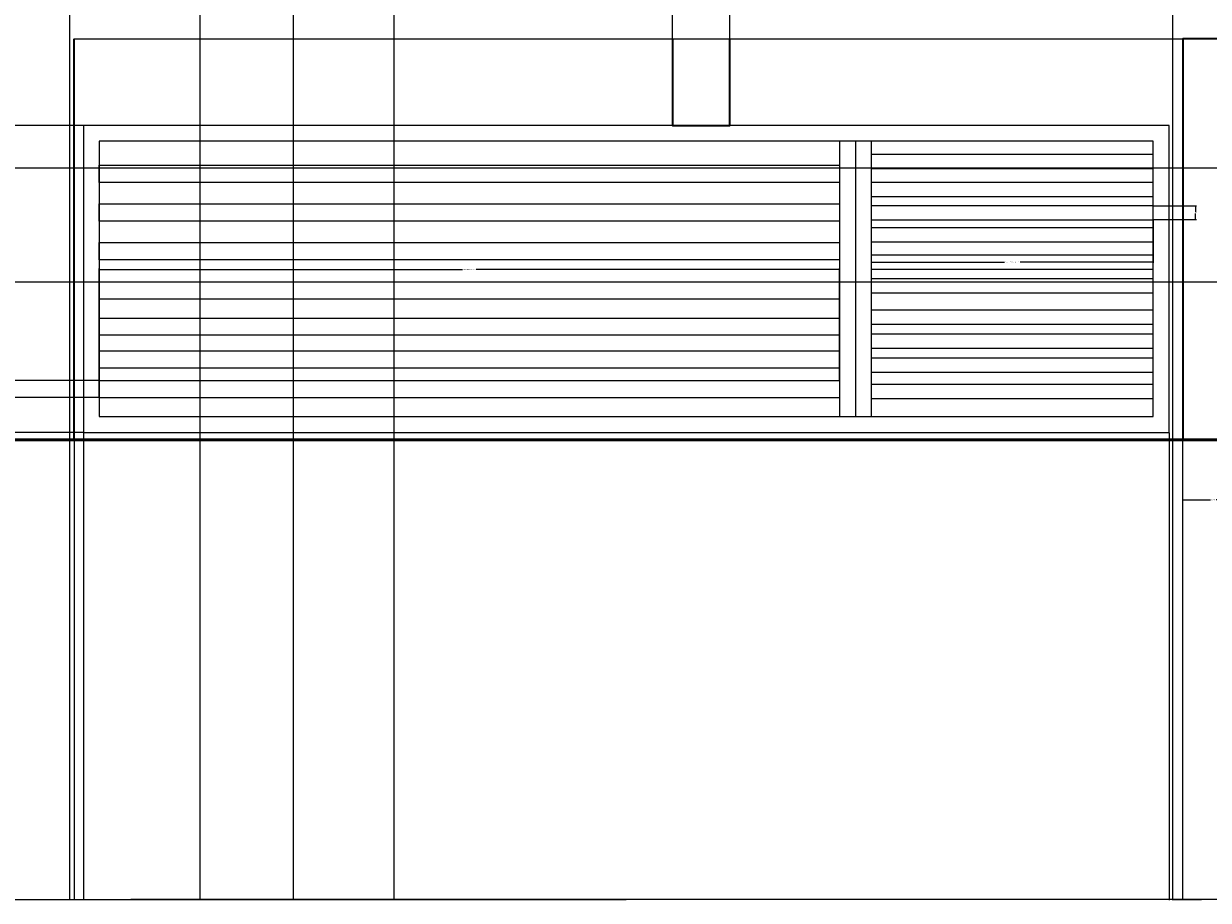
# Model space of a CAD drawing. Units: inches. Extents: x -8 to 554, y -200 to 499.
# Tile 3 of 12: x 214 to 439, y -200 to -34. Entities that reach past the tile are written whole.
import ezdxf

# ---------------------------------------------------------------- set-up
doc = ezdxf.new("R2010")
doc.units = ezdxf.units.IN
doc.header["$MEASUREMENT"] = 0
for name, color, linetype, lineweight in [('A-ANNO-DIMS', 2, 'Continuous', 18), ('A-COLS', 1, 'Continuous', 35), ('A-DOOR-GATE', 3, 'Continuous', 25), ('C-TOPO', 7, 'Continuous', 50)]:
    doc.layers.add(name, color=color, linetype=linetype, lineweight=lineweight)
doc.styles.get("Standard").update_dxf_attribs({"font": 'arial.ttf'})
doc.dimstyles.get("Standard").update_dxf_attribs({"dimtxt": 0.18, "dimasz": 0.18, "dimexe": 0.18, "dimexo": 0.0625, "dimgap": 0.09, "dimtad": 0, "dimtih": 1, "dimtoh": 1, "dimdec": 4, "dimzin": 0, "dimdsep": 46, "dimtxsty": 'Standard', "dimcen": 0.09, "dimadec": 0, "dimazin": 0, "dimtfac": 1, "dimtdec": 4, "dimtofl": 0, "dimtmove": 0, "dimatfit": 3, "dimfxl": 1, "dimtolj": 1, "dimtzin": 0, "dimarcsym": 0})

# ---------------------------------------------------------------- blocks, each defined once
blk = doc.blocks.new('GATE-PIER-ELEV')
blk.add_lwpolyline([(0, 76.14), (0, 0), (11.66, 0), (11.66, 76.14)])
blk = doc.blocks.new('GATE-SLAT-WIDE')
blk.add_lwpolyline([(0, 3.27), (140.62, 3.27), (140.62, 0), (0, 0)], close=True)
blk = doc.blocks.new('GATE-SLAT-NARROW')
blk.add_lwpolyline([(0, 0), (53.59, 0), (53.59, 2.66), (0, 2.66)], close=True)
blk = doc.blocks.new('*D12')
at = {"layer": 'A-ANNO-DIMS', "color": 0, "lineweight": -2, "transparency": 16777216}
for p, q in [((375.25, -70.8), (375.25, -78.95)), ((428.85, -70.8), (428.85, -78.95)), ((375.43, -78.77), (400.57, -78.77)), ((428.67, -78.77), (403.53, -78.77))]:
    blk.add_line(p, q, dxfattribs=at)
at = {"layer": 'A-ANNO-DIMS', "color": 0, "transparency": 16777216}
for points in [[(375.43, -78.74), (375.43, -78.8), (375.25, -78.77)], [(428.67, -78.74), (428.67, -78.8), (428.85, -78.77)]]:
    blk.add_solid(points, dxfattribs=at)
at = {"layer": 'Defpoints', "color": 0, "transparency": 16777216}
for p in [(375.25, -70.73), (428.85, -70.73), (428.85, -78.77)]:
    blk.add_point(p, dxfattribs=at)
at = {"layer": 'A-ANNO-DIMS', "color": 0, "transparency": 16777216, "insert": (402.05, -78.77), "char_height": 0.18, "attachment_point": 5}
blk.add_mtext('\\A1;NARROW SLAT 54 TYP.', dxfattribs=at)
blk = doc.blocks.new('*D13')
at = {"layer": 'A-ANNO-DIMS', "color": 0, "lineweight": -2, "transparency": 16777216}
for p, q in [((428.91, -68.08), (437.06, -68.08)), ((436.88, -68.26), (436.88, -69.22)), ((436.88, -70.55), (436.88, -69.59)), ((428.91, -70.73), (437.06, -70.73))]:
    blk.add_line(p, q, dxfattribs=at)
at = {"layer": 'A-ANNO-DIMS', "color": 0, "transparency": 16777216}
for points in [[(436.85, -68.26), (436.91, -68.26), (436.88, -68.08)], [(436.85, -70.55), (436.91, -70.55), (436.88, -70.73)]]:
    blk.add_solid(points, dxfattribs=at)
at = {"layer": 'Defpoints', "color": 0, "transparency": 16777216}
for p in [(428.85, -68.08), (436.88, -68.08), (428.85, -70.73)]:
    blk.add_point(p, dxfattribs=at)
at = {"layer": 'A-ANNO-DIMS', "color": 0, "transparency": 16777216, "insert": (436.88, -69.4), "char_height": 0.18, "attachment_point": 5}
blk.add_mtext('\\A1;3 TYP.', dxfattribs=at)
blk = doc.blocks.new('*D14')
at = {"layer": 'A-ANNO-DIMS', "color": 0, "lineweight": -2, "transparency": 16777216}
for p, q in [((228.63, -101.2), (228.63, -79.99)), ((228.81, -80.17), (297.63, -80.17)), ((369.07, -80.17), (300.26, -80.17)), ((369.25, -101.2), (369.25, -79.99))]:
    blk.add_line(p, q, dxfattribs=at)
at = {"layer": 'A-ANNO-DIMS', "color": 0, "transparency": 16777216}
for points in [[(228.81, -80.14), (228.81, -80.2), (228.63, -80.17)], [(369.07, -80.14), (369.07, -80.2), (369.25, -80.17)]]:
    blk.add_solid(points, dxfattribs=at)
at = {"layer": 'Defpoints', "color": 0, "transparency": 16777216}
for p in [(369.25, -80.17), (228.63, -101.26), (369.25, -101.26)]:
    blk.add_point(p, dxfattribs=at)
at = {"layer": 'A-ANNO-DIMS', "color": 0, "transparency": 16777216, "insert": (298.94, -80.17), "char_height": 0.18, "attachment_point": 5}
blk.add_mtext('\\A1;WIDE SLAT 141 TYP.', dxfattribs=at)
blk = doc.blocks.new('*D15')
at = {"layer": 'A-ANNO-DIMS', "color": 0, "lineweight": -2, "transparency": 16777216}
for p, q in [((228.57, -101.26), (207.36, -101.26)), ((207.54, -101.44), (207.54, -102.71)), ((207.54, -104.35), (207.54, -103.08)), ((228.57, -104.53), (207.36, -104.53))]:
    blk.add_line(p, q, dxfattribs=at)
at = {"layer": 'A-ANNO-DIMS', "color": 0, "transparency": 16777216}
for points in [[(207.51, -101.44), (207.57, -101.44), (207.54, -101.26)], [(207.51, -104.35), (207.57, -104.35), (207.54, -104.53)]]:
    blk.add_solid(points, dxfattribs=at)
at = {"layer": 'Defpoints', "color": 0, "transparency": 16777216}
for p in [(207.54, -101.26), (228.63, -101.26), (228.63, -104.53)]:
    blk.add_point(p, dxfattribs=at)
at = {"layer": 'A-ANNO-DIMS', "color": 0, "transparency": 16777216, "insert": (207.54, -102.9), "char_height": 0.18, "attachment_point": 5}
blk.add_mtext('\\A1;3 TYP.', dxfattribs=at)
blk = doc.blocks.new('*D29')
at = {"layer": 'A-ANNO-DIMS', "color": 0, "lineweight": -2, "transparency": 16777216}
for p, q in [((434.42, -112.58), (434.42, -124.12)), ((446.09, -112.58), (446.09, -124.12)), ((434.6, -123.94), (439.73, -123.94)), ((445.91, -123.94), (440.77, -123.94))]:
    blk.add_line(p, q, dxfattribs=at)
at = {"layer": 'A-ANNO-DIMS', "color": 0, "transparency": 16777216}
for points in [[(434.6, -123.91), (434.6, -123.97), (434.42, -123.94)], [(445.91, -123.91), (445.91, -123.97), (446.09, -123.94)]]:
    blk.add_solid(points, dxfattribs=at)
at = {"layer": 'Defpoints', "color": 0, "transparency": 16777216}
for p in [(434.42, -112.52), (446.09, -112.52), (434.42, -123.94)]:
    blk.add_point(p, dxfattribs=at)
at = {"layer": 'A-ANNO-DIMS', "color": 0, "transparency": 16777216, "insert": (440.25, -123.94), "char_height": 0.18, "attachment_point": 5}
blk.add_mtext('\\A1;12 TYP.', dxfattribs=at)
blk = doc.blocks.new('*D31')
at = {"layer": 'A-ANNO-DIMS', "color": 0, "lineweight": -2, "transparency": 16777216}
for p, q in [((24.34, 127.42), (24.34, -199.97)), ((453.32, -30.73), (453.32, -199.97)), ((24.52, -199.79), (238.54, -199.79)), ((453.14, -199.79), (239.12, -199.79))]:
    blk.add_line(p, q, dxfattribs=at)
at = {"layer": 'A-ANNO-DIMS', "color": 0, "transparency": 16777216}
for points in [[(24.52, -199.76), (24.52, -199.82), (24.34, -199.79)], [(453.14, -199.76), (453.14, -199.82), (453.32, -199.79)]]:
    blk.add_solid(points, dxfattribs=at)
at = {"layer": 'Defpoints', "color": 0, "transparency": 16777216}
for p in [(24.34, 127.48), (453.32, -30.67), (453.32, -199.79)]:
    blk.add_point(p, dxfattribs=at)
at = {"layer": 'A-ANNO-DIMS', "color": 0, "transparency": 16777216, "insert": (238.83, -199.79), "char_height": 0.18, "attachment_point": 5}
blk.add_mtext('\\A1;429', dxfattribs=at)
blk = doc.blocks.new('*D32')
at = {"layer": 'A-ANNO-DIMS', "color": 0, "lineweight": -2, "transparency": 16777216}
for p, q in [((24.34, 223.42), (24.34, -199.97)), ((444.34, 223.42), (444.34, -199.97)), ((24.52, -199.79), (234.05, -199.79)), ((444.16, -199.79), (234.63, -199.79))]:
    blk.add_line(p, q, dxfattribs=at)
at = {"layer": 'A-ANNO-DIMS', "color": 0, "transparency": 16777216}
for points in [[(24.52, -199.76), (24.52, -199.82), (24.34, -199.79)], [(444.16, -199.76), (444.16, -199.82), (444.34, -199.79)]]:
    blk.add_solid(points, dxfattribs=at)
at = {"layer": 'Defpoints', "color": 0, "transparency": 16777216}
for p in [(24.34, 223.48), (444.34, 223.48), (444.34, -199.79)]:
    blk.add_point(p, dxfattribs=at)
at = {"layer": 'A-ANNO-DIMS', "color": 0, "transparency": 16777216, "insert": (234.34, -199.79), "char_height": 0.18, "attachment_point": 5}
blk.add_mtext('\\A1;420', dxfattribs=at)
blk = doc.blocks.new('*D53')
at = {"layer": 'A-ANNO-DIMS', "color": 0, "lineweight": -2, "transparency": 16777216}
for p, q in [((223.89, -112.58), (223.89, -199.97)), ((434.42, -112.58), (434.42, -199.97)), ((224.07, -199.79), (328.69, -199.79)), ((434.24, -199.79), (329.62, -199.79))]:
    blk.add_line(p, q, dxfattribs=at)
at = {"layer": 'A-ANNO-DIMS', "color": 0, "transparency": 16777216}
for points in [[(224.07, -199.76), (224.07, -199.82), (223.89, -199.79)], [(434.24, -199.76), (434.24, -199.82), (434.42, -199.79)]]:
    blk.add_solid(points, dxfattribs=at)
at = {"layer": 'Defpoints', "color": 0, "transparency": 16777216}
for p in [(223.89, -112.52), (434.42, -112.52), (434.42, -199.79)]:
    blk.add_point(p, dxfattribs=at)
at = {"layer": 'A-ANNO-DIMS', "color": 0, "transparency": 16777216, "insert": (329.16, -199.79), "char_height": 0.18, "attachment_point": 5}
blk.add_mtext('\\A1;210.53', dxfattribs=at)
blk = doc.blocks.new('*D63')
at = {"layer": 'A-ANNO-DIMS', "color": 0, "lineweight": -2, "transparency": 16777216}
for p, q in [((337.49, -52.76), (337.49, 498.99)), ((337.67, 498.81), (342.51, 498.81)), ((348.26, 498.81), (343.42, 498.81)), ((348.44, -52.76), (348.44, 498.99))]:
    blk.add_line(p, q, dxfattribs=at)
at = {"layer": 'A-ANNO-DIMS', "color": 0, "transparency": 16777216}
for points in [[(337.67, 498.84), (337.67, 498.78), (337.49, 498.81)], [(348.26, 498.84), (348.26, 498.78), (348.44, 498.81)]]:
    blk.add_solid(points, dxfattribs=at)
at = {"layer": 'Defpoints', "color": 0, "transparency": 16777216}
for p in [(348.44, 498.81), (337.49, -52.82), (348.44, -52.82)]:
    blk.add_point(p, dxfattribs=at)
at = {"layer": 'A-ANNO-DIMS', "color": 0, "transparency": 16777216, "insert": (342.97, 498.81), "char_height": 0.18, "attachment_point": 5}
blk.add_mtext('\\A1;10.946', dxfattribs=at)
blk = doc.blocks.new('*D66')
at = {"layer": 'A-ANNO-DIMS', "color": 0, "lineweight": -2, "transparency": 16777216}
for p, q in [((225.57, -52.82), (-7.69, -52.82)), ((-7.51, -53), (-7.51, -81.79)), ((-7.51, -110.95), (-7.51, -82.16)), ((225.57, -111.13), (-7.69, -111.13))]:
    blk.add_line(p, q, dxfattribs=at)
at = {"layer": 'A-ANNO-DIMS', "color": 0, "transparency": 16777216}
for points in [[(-7.54, -53), (-7.48, -53), (-7.51, -52.82)], [(-7.54, -110.95), (-7.48, -110.95), (-7.51, -111.13)]]:
    blk.add_solid(points, dxfattribs=at)
at = {"layer": 'Defpoints', "color": 0, "transparency": 16777216}
for p in [(225.63, -52.82), (-7.51, -111.13), (225.63, -111.13)]:
    blk.add_point(p, dxfattribs=at)
at = {"layer": 'A-ANNO-DIMS', "color": 0, "transparency": 16777216, "insert": (-7.51, -81.98), "char_height": 0.18, "attachment_point": 5}
blk.add_mtext('\\A1;58.3', dxfattribs=at)
blk = doc.blocks.new('*D67')
at = {"layer": 'A-ANNO-DIMS', "color": 0, "lineweight": -2, "transparency": 16777216}
for p, q in [((223.01, 427.42), (223.01, -199.97)), ((247.72, 427.42), (247.72, -199.97)), ((223.19, -199.79), (234.9, -199.79)), ((247.54, -199.79), (235.83, -199.79))]:
    blk.add_line(p, q, dxfattribs=at)
at = {"layer": 'A-ANNO-DIMS', "color": 0, "transparency": 16777216}
for points in [[(223.19, -199.76), (223.19, -199.82), (223.01, -199.79)], [(247.54, -199.76), (247.54, -199.82), (247.72, -199.79)]]:
    blk.add_solid(points, dxfattribs=at)
at = {"layer": 'Defpoints', "color": 0, "transparency": 16777216}
for p in [(223.01, 427.48), (247.72, 427.48), (247.72, -199.79)]:
    blk.add_point(p, dxfattribs=at)
at = {"layer": 'A-ANNO-DIMS', "color": 0, "transparency": 16777216, "insert": (235.36, -199.79), "char_height": 0.18, "attachment_point": 5}
blk.add_mtext('\\A1;24.705', dxfattribs=at)
blk = doc.blocks.new('*D68')
at = {"layer": 'A-ANNO-DIMS', "color": 0, "lineweight": -2, "transparency": 16777216}
for p, q in [((247.72, 371.73), (247.72, -199.97)), ((265.46, 371.73), (265.46, -199.97)), ((247.9, -199.79), (256.13, -199.79)), ((265.28, -199.79), (257.04, -199.79))]:
    blk.add_line(p, q, dxfattribs=at)
at = {"layer": 'A-ANNO-DIMS', "color": 0, "transparency": 16777216}
for points in [[(247.9, -199.76), (247.9, -199.82), (247.72, -199.79)], [(265.28, -199.76), (265.28, -199.82), (265.46, -199.79)]]:
    blk.add_solid(points, dxfattribs=at)
at = {"layer": 'Defpoints', "color": 0, "transparency": 16777216}
for p in [(247.72, 371.79), (265.46, 371.79), (265.46, -199.79)]:
    blk.add_point(p, dxfattribs=at)
at = {"layer": 'A-ANNO-DIMS', "color": 0, "transparency": 16777216, "insert": (256.59, -199.79), "char_height": 0.18, "attachment_point": 5}
blk.add_mtext('\\A1;17.744', dxfattribs=at)
blk = doc.blocks.new('*D69')
at = {"layer": 'A-ANNO-DIMS', "color": 0, "lineweight": -2, "transparency": 16777216}
for p, q in [((265.46, 371.73), (265.46, -199.97)), ((284.57, 371.73), (284.57, -199.97)), ((265.64, -199.79), (274.65, -199.79)), ((284.39, -199.79), (275.38, -199.79))]:
    blk.add_line(p, q, dxfattribs=at)
at = {"layer": 'A-ANNO-DIMS', "color": 0, "transparency": 16777216}
for points in [[(265.64, -199.76), (265.64, -199.82), (265.46, -199.79)], [(284.39, -199.76), (284.39, -199.82), (284.57, -199.79)]]:
    blk.add_solid(points, dxfattribs=at)
at = {"layer": 'Defpoints', "color": 0, "transparency": 16777216}
for p in [(265.46, 371.79), (284.57, 371.79), (284.57, -199.79)]:
    blk.add_point(p, dxfattribs=at)
at = {"layer": 'A-ANNO-DIMS', "color": 0, "transparency": 16777216, "insert": (275.01, -199.79), "char_height": 0.18, "attachment_point": 5}
blk.add_mtext('\\A1;19.11', dxfattribs=at)
blk = doc.blocks.new('*D71')
at = {"layer": 'A-ANNO-DIMS', "color": 0, "lineweight": -2, "transparency": 16777216}
for p, q in [((444.34, 439.42), (444.34, -199.97)), ((432.52, 427.42), (432.52, -199.97)), ((432.7, -199.79), (437.97, -199.79)), ((444.16, -199.79), (438.89, -199.79))]:
    blk.add_line(p, q, dxfattribs=at)
at = {"layer": 'A-ANNO-DIMS', "color": 0, "transparency": 16777216}
for points in [[(432.7, -199.76), (432.7, -199.82), (432.52, -199.79)], [(444.16, -199.76), (444.16, -199.82), (444.34, -199.79)]]:
    blk.add_solid(points, dxfattribs=at)
at = {"layer": 'Defpoints', "color": 0, "transparency": 16777216}
for p in [(444.34, 439.48), (432.52, 427.48), (444.34, -199.79)]:
    blk.add_point(p, dxfattribs=at)
at = {"layer": 'A-ANNO-DIMS', "color": 0, "transparency": 16777216, "insert": (438.43, -199.79), "char_height": 0.18, "attachment_point": 5}
blk.add_mtext('\\A1;11.825', dxfattribs=at)
blk = doc.blocks.new('*D76')
at = {"layer": 'A-ANNO-DIMS', "color": 0, "lineweight": -2, "transparency": 16777216}
for p, q in [((48.75, -82.52), (554.26, -82.52)), ((554.08, -82.7), (554.08, -97.34)), ((554.08, -112.34), (554.08, -97.7)), ((48.75, -112.52), (554.26, -112.52))]:
    blk.add_line(p, q, dxfattribs=at)
at = {"layer": 'A-ANNO-DIMS', "color": 0, "transparency": 16777216}
for points in [[(554.05, -82.7), (554.11, -82.7), (554.08, -82.52)], [(554.05, -112.34), (554.11, -112.34), (554.08, -112.52)]]:
    blk.add_solid(points, dxfattribs=at)
at = {"layer": 'Defpoints', "color": 0, "transparency": 16777216}
for p in [(48.69, -82.52), (554.08, -82.52), (48.69, -112.52)]:
    blk.add_point(p, dxfattribs=at)
at = {"layer": 'A-ANNO-DIMS', "color": 0, "transparency": 16777216, "insert": (554.08, -97.52), "char_height": 0.18, "attachment_point": 5}
blk.add_mtext('\\A1;30', dxfattribs=at)
blk = doc.blocks.new('*D77')
at = {"layer": 'A-ANNO-DIMS', "color": 0, "lineweight": -2, "transparency": 16777216}
for p, q in [((48.75, -60.9), (554.26, -60.9)), ((554.08, -61.08), (554.08, -71.53)), ((554.08, -82.34), (554.08, -71.89)), ((48.75, -82.52), (554.26, -82.52))]:
    blk.add_line(p, q, dxfattribs=at)
at = {"layer": 'A-ANNO-DIMS', "color": 0, "transparency": 16777216}
for points in [[(554.05, -61.08), (554.11, -61.08), (554.08, -60.9)], [(554.05, -82.34), (554.11, -82.34), (554.08, -82.52)]]:
    blk.add_solid(points, dxfattribs=at)
at = {"layer": 'Defpoints', "color": 0, "transparency": 16777216}
for p in [(48.69, -60.9), (554.08, -60.9), (48.69, -82.52)]:
    blk.add_point(p, dxfattribs=at)
at = {"layer": 'A-ANNO-DIMS', "color": 0, "transparency": 16777216, "insert": (554.08, -71.71), "char_height": 0.18, "attachment_point": 5}
blk.add_mtext('\\A1;21.615', dxfattribs=at)
blk = doc.blocks.new('*D79')
at = {"layer": 'A-ANNO-DIMS', "color": 0, "lineweight": -2, "transparency": 16777216}
for p, q in [((225.63, -111.19), (225.63, -199.97)), ((431.85, -111.19), (431.85, -199.97)), ((225.81, -199.79), (328.34, -199.79)), ((431.67, -199.79), (329.13, -199.79))]:
    blk.add_line(p, q, dxfattribs=at)
at = {"layer": 'A-ANNO-DIMS', "color": 0, "transparency": 16777216}
for points in [[(225.81, -199.76), (225.81, -199.82), (225.63, -199.79)], [(431.67, -199.76), (431.67, -199.82), (431.85, -199.79)]]:
    blk.add_solid(points, dxfattribs=at)
at = {"layer": 'Defpoints', "color": 0, "transparency": 16777216}
for p in [(225.63, -111.13), (431.85, -111.13), (431.85, -199.79)]:
    blk.add_point(p, dxfattribs=at)
at = {"layer": 'A-ANNO-DIMS', "color": 0, "transparency": 16777216, "insert": (328.74, -199.79), "char_height": 0.18, "attachment_point": 5}
blk.add_mtext('\\A1;206.2', dxfattribs=at)

msp = doc.modelspace()

# ---------------------------------------------------------------- linework, layer by layer
at = {"layer": 'A-COLS'}
msp.add_lwpolyline([(337.4923, -36.3739), (337.4923, -52.8232), (348.4381, -52.8232), (348.4381, -36.3739)], dxfattribs=at)
at = {"layer": 'A-DOOR-GATE'}
for p, q in [((369.2536, -55.8232), (369.2536, -108.1275)), ((372.2536, -55.8232), (372.2536, -108.1275)), ((375.2536, -55.8232), (375.2536, -108.1275))]:
    msp.add_line(p, q, dxfattribs=at)
msp.add_lwpolyline([(223.8912, -36.3739), (434.4225, -36.3739)], dxfattribs=at)
for points in [[(225.6322, -111.1275), (431.8451, -111.1275), (431.8451, -52.8232), (225.6322, -52.8232)], [(228.6322, -108.1275), (428.8451, -108.1275), (428.8451, -55.8232), (228.6322, -55.8232)]]:
    msp.add_lwpolyline(points, close=True, dxfattribs=at)
at = {"layer": 'C-TOPO'}
msp.add_line((24.3421, -112.5186), (522.2333, -112.5186), dxfattribs=at)

# ---------------------------------------------------------------- block references
at = {"layer": 'A-COLS'}
msp.add_blockref('GATE-PIER-ELEV', (212.2282, -112.5186), dxfattribs=at)
at = {"layer": 'A-COLS', "rotation": 180}
msp.add_blockref('GATE-PIER-ELEV', (446.0855, -36.3739), dxfattribs=at)
at = {"layer": 'A-DOOR-GATE'}
for name, p in [('GATE-SLAT-NARROW', (375.2536, -61.038)), ('GATE-SLAT-WIDE', (228.6322, -63.6625)), ('GATE-SLAT-NARROW', (375.2536, -66.3551)), ('GATE-SLAT-WIDE', (228.6322, -71.0215)), ('GATE-SLAT-NARROW', (375.2536, -70.7338)), ('GATE-SLAT-NARROW', (375.2536, -74.9561)), ('GATE-SLAT-WIDE', (228.6322, -78.347)), ('GATE-SLAT-NARROW', (375.2536, -80.1168)), ('GATE-SLAT-WIDE', (228.6322, -85.8285)), ('GATE-SLAT-NARROW', (375.2536, -84.6338)), ('GATE-SLAT-WIDE', (228.6322, -92.6864)), ('GATE-SLAT-NARROW', (375.2536, -90.5944)), ('GATE-SLAT-NARROW', (375.2536, -95.1295)), ('GATE-SLAT-WIDE', (228.6322, -98.9209)), ('GATE-SLAT-NARROW', (375.2536, -99.6647)), ('GATE-SLAT-WIDE', (228.6322, -104.532)), ('GATE-SLAT-NARROW', (375.2536, -104.6689))]:
    msp.add_blockref(name, p, dxfattribs=at)

# ---------------------------------------------------------------- dimensions: what is measured, and where the dimension line sits
at = {"layer": 'A-ANNO-DIMS'}
for base, p1, p2, override, picture, middle in [((348.4381, 498.8091), (337.4923, -52.8232), (348.4381, -52.8232), {"dimdec": 3, "dimlfac": 1, "dimrnd": 0, "dimzin": 0, "dimdsep": 46, "dimlunit": 2}, '*D63', (342.9652, 498.8091)), ((444.3421, -199.7912), (432.5174, 427.4814), (444.3421, 439.4814), {"dimdec": 3, "dimlfac": 1, "dimrnd": 0, "dimzin": 0, "dimdsep": 46, "dimlunit": 2}, '*D71', (438.4297, -199.7912)), ((247.71587, -199.79119), (223.01039, 427.48136), (247.71587, 427.48136), {"dimdec": 3, "dimlfac": 1, "dimrnd": 0, "dimzin": 0, "dimdsep": 46, "dimlunit": 2}, '*D67', (235.36313, -199.79119)), ((265.4598, -199.7912), (247.7159, 371.7921), (265.4598, 371.7921), {"dimdec": 3, "dimlfac": 1, "dimrnd": 0, "dimzin": 0, "dimdsep": 46, "dimlunit": 2}, '*D68', (256.5878, -199.7912)), ((284.5686, -199.7912), (265.4598, 371.7921), (284.5686, 371.7921), {"dimdec": 2, "dimlfac": 1, "dimrnd": 0, "dimzin": 0, "dimdsep": 46, "dimlunit": 2}, '*D69', (275.0142, -199.7912)), ((444.3421, -199.7912), (24.3421, 223.4814), (444.3421, 223.4814), {"dimdec": 0, "dimlfac": 1, "dimrnd": 0, "dimzin": 0, "dimdsep": 46, "dimlunit": 2}, '*D32', (234.3421, -199.7912)), ((453.3222, -199.7912), (24.3421, 127.4814), (453.3222, -30.6677), {"dimdec": 0, "dimlfac": 1, "dimrnd": 0, "dimzin": 0, "dimdsep": 46, "dimlunit": 2}, '*D31', (238.8321, -199.7912)), ((431.8451, -199.7912), (225.6322, -111.1275), (431.8451, -111.1275), {"dimdec": 1, "dimlfac": 1, "dimrnd": 0, "dimzin": 0, "dimdsep": 46, "dimlunit": 2}, '*D79', (328.7386, -199.7912)), ((434.4225, -199.7912), (223.8912, -112.5186), (434.4225, -112.5186), {"dimdec": 2, "dimlfac": 1, "dimrnd": 0, "dimzin": 0, "dimdsep": 46, "dimlunit": 2}, '*D53', (329.1568, -199.7912))]:
    dim = msp.add_linear_dim(base=base, p1=p1, p2=p2, dimstyle='Standard', override=override, dxfattribs=at)
    dim.commit()
    dim.dimension.update_dxf_attribs({"geometry": picture, "text_midpoint": middle})
for base, p1, p2, override, picture, middle in [((-7.5079, -111.1275), (225.6322, -52.8232), (225.6322, -111.1275), {"dimdec": 1, "dimlfac": 1, "dimrnd": 0, "dimzin": 0, "dimdsep": 46, "dimlunit": 2}, '*D66', (-7.5079, -81.9753)), ((554.0833, -60.9032), (48.6882, -82.5186), (48.6882, -60.9032), {"dimdec": 3, "dimlfac": 1, "dimrnd": 0, "dimzin": 0, "dimdsep": 46, "dimlunit": 2}, '*D77', (554.0833, -71.7109)), ((554.0833, -82.5186), (48.6882, -112.5186), (48.6882, -82.5186), {"dimdec": 0, "dimlfac": 1, "dimrnd": 0, "dimzin": 0, "dimdsep": 46, "dimlunit": 2}, '*D76', (554.0833, -97.5186))]:
    dim = msp.add_linear_dim(base=base, p1=p1, p2=p2, angle=90, dimstyle='Standard', override=override, dxfattribs=at)
    dim.commit()
    dim.dimension.update_dxf_attribs({"geometry": picture, "text_midpoint": middle})
for base, p1, p2, angle, picture, middle in [((436.8838, -68.0753), (428.8451, -70.7338), (428.8451, -68.0753), 90, '*D13', (436.8838, -69.4045)), ((207.539, -101.2589), (228.6322, -104.532), (228.6322, -101.2589), 90, '*D15', (207.539, -102.8954)), ((434.4225, -123.9404), (446.0855, -112.5186), (434.4225, -112.5186), 180, '*D29', (440.254, -123.9404))]:
    dim = msp.add_linear_dim(base=base, p1=p1, p2=p2, angle=angle, text='<> TYP.', dimstyle='Standard', override={"dimdec": 0, "dimlfac": 1, "dimrnd": 0, "dimzin": 0, "dimdsep": 46, "dimlunit": 2}, dxfattribs=at)
    dim.commit()
    dim.dimension.update_dxf_attribs({"geometry": picture, "text_midpoint": middle})
for base, p1, p2, text, picture, middle in [((428.8451, -78.7725), (375.2536, -70.7338), (428.8451, -70.7338), 'NARROW SLAT <> TYP.', '*D12', (402.0493, -78.7725)), ((369.2536, -80.1657), (228.6322, -101.2589), (369.2536, -101.2589), 'WIDE SLAT <> TYP.', '*D14', (298.9429, -80.1657))]:
    dim = msp.add_linear_dim(base=base, p1=p1, p2=p2, text=text, dimstyle='Standard', override={"dimdec": 0, "dimlfac": 1, "dimrnd": 0, "dimzin": 0, "dimdsep": 46, "dimlunit": 2}, dxfattribs=at)
    dim.commit()
    dim.dimension.update_dxf_attribs({"geometry": picture, "text_midpoint": middle})

doc.saveas('drawing.dxf')
